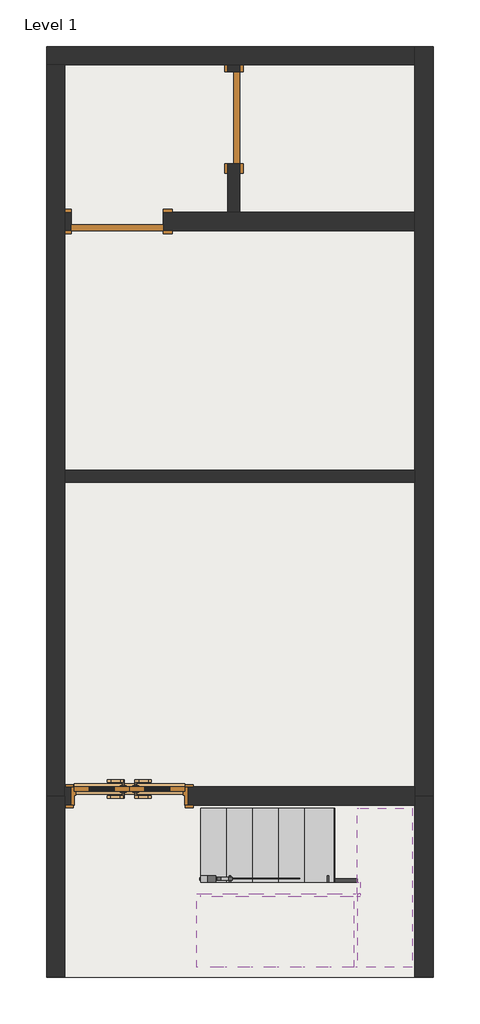
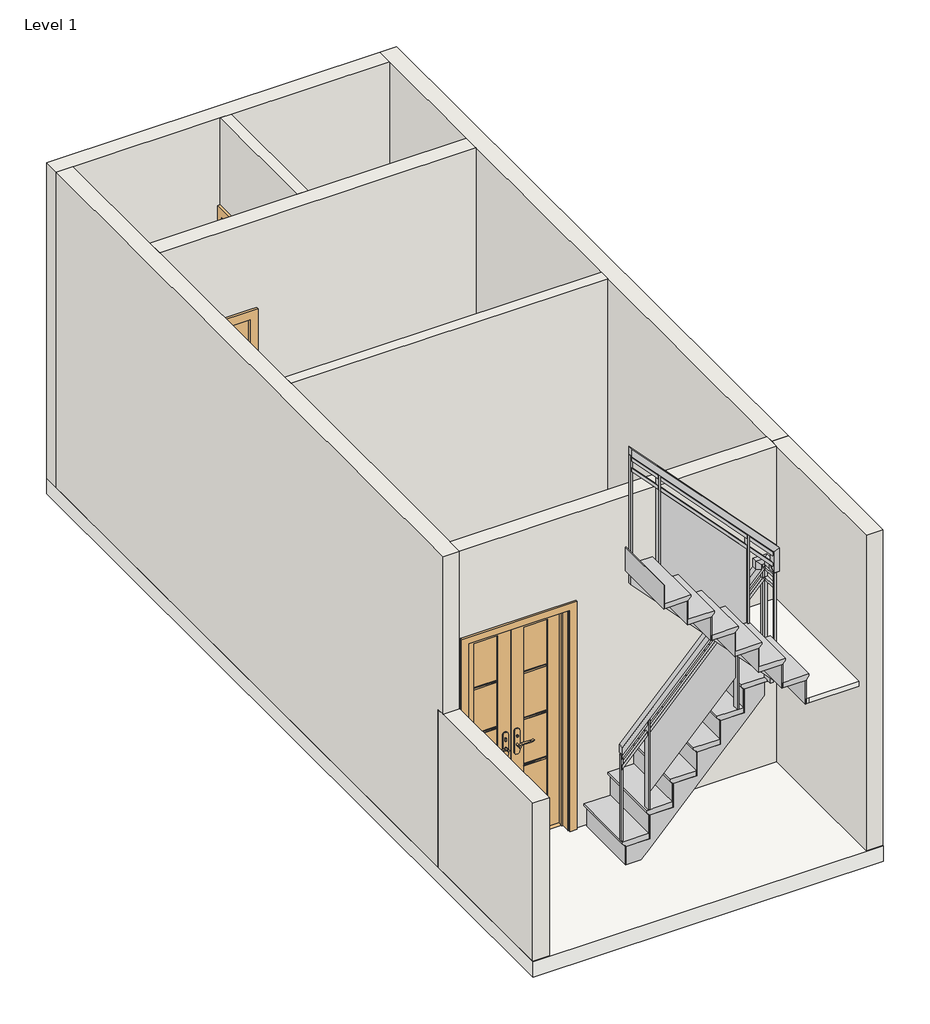
# One storey: 9 walls, 3 doors, 3 members, 2 slabs, 2 stair flights, 1 railing.
"""IFC4 building model written with IfcOpenShell, lengths in millimetres."""

from ifc_helpers import new_model, si_unit, frame, origin, origin_with_axes, place, context, project, spatial, polyline, outline, extrude, faceted_brep, transform, mapped, element, save
from components import door_665efd91, single_flush_2_5_a9addea7, single_flush_2_5_aa9e95e7, non_monolithic_landing_a944a33a, stair_flight_4ab14130, stair_flight_03d0a82c

model = new_model("IFC4")

# Units and contexts
model_context = context("Model", 3, world=origin())
ifc_project = project(units=[si_unit("LENGTHUNIT", "METRE", prefix="MILLI")], contexts=[model_context])

# Site, building, storey
site = spatial("IfcSite", under=ifc_project)
building = spatial("IfcBuilding", under=site)
storey = spatial("IfcBuildingStorey", under=building, Name="Level 1", Elevation=0.0)

# Doors
placement = place(None, origin())
door_shape = door_665efd91(model_context)
element("IfcDoor", 1, ObjectType="Door-Exterior-Double-Full Glass-Wood_Clad : 60\" x 84\"", at=placement, inside=storey, context=model_context, shape_type="MappedRepresentation", body=[
    mapped(door_shape, transform((-5617.280937, -3133.7029636, 0.0), x_axis=(1.0, 0.0, 0.0), y_axis=(0.0, 1.0, 0.0), z_axis=(0.0, 0.0, 1.0))),
])
single_flush_2_5_shape = single_flush_2_5_a9addea7(model_context)
element("IfcDoor", 2, ObjectType="Single-Flush : 2.5'", at=placement, inside=storey, context=model_context, shape_type="MappedRepresentation", body=[
    mapped(single_flush_2_5_shape, transform((-5718.880937, 1617.2335625, 0.0), x_axis=(-1.0, 0.0, 0.0), y_axis=(0.0, -1.0, 0.0), z_axis=(0.0, 0.0, 1.0))),
])
single_flush_2_5_2_shape = single_flush_2_5_aa9e95e7(model_context)
element("IfcDoor", 3, ObjectType="Single-Flush : 2.5'", at=placement, inside=storey, context=model_context, shape_type="MappedRepresentation", body=[
    mapped(single_flush_2_5_2_shape, transform((-4753.680937, 2474.4835625, 0.0), x_axis=(0.0, 1.0, 0.0), y_axis=(-1.0, 0.0, 0.0), z_axis=(0.0, 0.0, 1.0))),
])

# Members
element("IfcMember", 4, ObjectType="Carriage - 2\" Width", at=placement, inside=storey, context=model_context, shape_type="Brep", body=[
    faceted_brep([(-4996.3909298, -3822.6779636, 0.0), (-4861.0694778, -3822.6779636, 0.0), (-4861.0694778, -3848.0779636, 0.0), (-4996.3909298, -3848.0779636, 0.0), (-3732.7409298, -3822.6779636, 1194.7008155), (-3732.7409298, -3848.0779636, 1194.7008155), (-3916.8909298, -3848.0779636, 999.7184625), (-4132.7909298, -3848.0779636, 771.1184625), (-4348.6909298, -3848.0779636, 542.5184625), (-4564.5909298, -3848.0779636, 313.9184625), (-4780.4909298, -3848.0779636, 85.3184625), (-3732.7409298, -3822.6779636, 1320.8), (-4996.3909298, -3822.6779636, 177.8), (-4780.4909298, -3822.6779636, 177.8), (-4780.4909298, -3822.6779636, 406.4), (-4564.5909298, -3822.6779636, 406.4), (-4564.5909298, -3822.6779636, 635.0), (-4348.6909298, -3822.6779636, 635.0), (-4348.6909298, -3822.6779636, 863.6), (-4132.7909298, -3822.6779636, 863.6), (-4132.7909298, -3822.6779636, 1092.2), (-3916.8909298, -3822.6779636, 1092.2), (-3916.8909298, -3822.6779636, 1320.8), (-3916.8909298, -3848.0779636, 1320.8), (-3732.7409298, -3848.0779636, 1320.8), (-3916.8909298, -3848.0779636, 1092.2), (-4132.7909298, -3848.0779636, 1092.2), (-4132.7909298, -3848.0779636, 863.6), (-4348.6909298, -3848.0779636, 863.6), (-4348.6909298, -3848.0779636, 635.0), (-4564.5909298, -3848.0779636, 635.0), (-4564.5909298, -3848.0779636, 406.4), (-4780.4909298, -3848.0779636, 406.4), (-4780.4909298, -3848.0779636, 177.8), (-4996.3909298, -3848.0779636, 177.8)], [[[0, 1, 2, 3]], [[4, 5, 6, 7, 8, 9, 10, 2, 1]], [[11, 4, 1, 0, 12, 13, 14, 15, 16, 17, 18, 19, 20, 21, 22]], [[22, 23, 24, 11]], [[5, 24, 23, 25, 26, 27, 28, 29, 30, 31, 32, 33, 34, 3, 2, 10, 9, 8, 7, 6]], [[34, 12, 0, 3]], [[12, 34, 33, 13]], [[13, 33, 32, 14]], [[14, 32, 31, 15]], [[15, 31, 30, 16]], [[16, 30, 29, 17]], [[17, 29, 28, 18]], [[18, 28, 27, 19]], [[19, 27, 26, 20]], [[20, 26, 25, 21]], [[21, 25, 23, 22]], [[5, 4, 11, 24]]]),
])
element("IfcMember", 5, ObjectType="Carriage - 2\" Width", at=placement, inside=storey, context=model_context, shape_type="Brep", body=[
    faceted_brep([(-5028.1409298, -3945.3664375, 2794.9008155), (-5028.1409298, -3970.7664375, 2794.9008155), (-5028.1409298, -3970.7664375, 2921.0), (-5028.1409298, -3945.3664375, 2921.0), (-3707.3409298, -3970.7664375, 1396.4066978), (-3707.3409298, -3970.7664375, 1549.4), (-3764.4909298, -3970.7664375, 1549.4), (-3764.4909298, -3970.7664375, 1778.0), (-3980.3909298, -3970.7664375, 1778.0), (-3980.3909298, -3970.7664375, 2006.6), (-4196.2909298, -3970.7664375, 2006.6), (-4196.2909298, -3970.7664375, 2235.2), (-4412.1909298, -3970.7664375, 2235.2), (-4412.1909298, -3970.7664375, 2463.8), (-4628.0909298, -3970.7664375, 2463.8), (-4628.0909298, -3970.7664375, 2692.4), (-4843.9909298, -3970.7664375, 2692.4), (-4843.9909298, -3970.7664375, 2921.0), (-4843.9909298, -3945.3664375, 2599.9184625), (-4628.0909298, -3945.3664375, 2371.3184625), (-4412.1909298, -3945.3664375, 2142.7184625), (-4196.2909298, -3945.3664375, 1914.1184625), (-3980.3909298, -3945.3664375, 1685.5184625), (-3764.4909298, -3945.3664375, 1456.9184625), (-3732.7409298, -3945.3664375, 1423.3008155), (-3707.3409298, -3945.3664375, 1396.4066978), (-4843.9909298, -3945.3664375, 2921.0), (-4843.9909298, -3945.3664375, 2692.4), (-4628.0909298, -3945.3664375, 2692.4), (-4628.0909298, -3945.3664375, 2463.8), (-4412.1909298, -3945.3664375, 2463.8), (-4412.1909298, -3945.3664375, 2235.2), (-4196.2909298, -3945.3664375, 2235.2), (-4196.2909298, -3945.3664375, 2006.6), (-3980.3909298, -3945.3664375, 2006.6), (-3980.3909298, -3945.3664375, 1778.0), (-3764.4909298, -3945.3664375, 1778.0), (-3764.4909298, -3945.3664375, 1549.4), (-3732.7409298, -3945.3664375, 1549.4), (-3707.3409298, -3945.3664375, 1549.4)], [[[0, 1, 2, 3]], [[1, 4, 5, 6, 7, 8, 9, 10, 11, 12, 13, 14, 15, 16, 17, 2]], [[1, 0, 18, 19, 20, 21, 22, 23, 24, 25, 4]], [[0, 3, 26, 27, 28, 29, 30, 31, 32, 33, 34, 35, 36, 37, 38, 39, 25, 24, 23, 22, 21, 20, 19, 18]], [[7, 36, 35, 8]], [[36, 7, 6, 37]], [[9, 34, 33, 10]], [[8, 35, 34, 9]], [[11, 32, 31, 12]], [[10, 33, 32, 11]], [[13, 30, 29, 14]], [[12, 31, 30, 13]], [[15, 28, 27, 16]], [[14, 29, 28, 15]], [[17, 26, 3, 2]], [[16, 27, 26, 17]], [[4, 25, 39, 5]], [[37, 6, 5, 39, 38]]]),
])
element("IfcMember", 6, ObjectType="Carriage - 2\" Width", at=placement, inside=storey, context=model_context, shape_type="SweptSolid", body=[
    extrude(outline(polyline([(-3707.3409298, -3945.3664375), (-3732.7409298, -3945.3664375), (-3732.7409298, -3848.0779636), (-3707.3409298, -3848.0779636), (-3707.3409298, -3945.3664375)])), frame((0.0, 0.0, 1371.6), z_axis=(0.0, 0.0, 1.0), x_axis=(1.0, 0.0, 0.0)), (0.0, 0.0, 1.0), 177.8),
])

# Railing
element("IfcRailing", 7, ObjectType="Glass Panel - Bottom Fill", at=placement, inside=storey, context=model_context, shape_type="SolidModel", body=[
    faceted_brep([(-5028.1409298, -3797.2779636, 1143.0), (-5028.1409298, -3797.2779636, 1069.01477), (-5028.1409298, -3848.0779636, 1069.01477), (-5028.1409298, -3848.0779636, 1143.0), (-3808.9409298, -3797.2779636, 2433.9176471), (-3758.1409298, -3797.2779636, 2413.7206524), (-3758.1409298, -3848.0779636, 2413.7206524), (-3808.9409298, -3848.0779636, 2433.9176471), (-3681.9409298, -3945.3664375, 2514.6), (-3732.7409298, -3945.3664375, 2514.6), (-3732.7409298, -3996.1664375, 2463.8), (-3681.9409298, -3996.1664375, 2463.8), (-3681.9409298, -3924.2779636, 2463.8), (-3681.9409298, -3924.2779636, 2514.6), (-3732.7409298, -3924.2779636, 2463.8), (-3732.7409298, -3924.2779636, 2514.6), (-3808.9409298, -3797.2779636, 2514.6), (-3758.1409298, -3797.2779636, 2463.8), (-3758.1409298, -3848.0779636, 2463.8), (-3808.9409298, -3848.0779636, 2514.6), (-3681.9409298, -3797.2779636, 2514.6), (-3681.9409298, -3797.2779636, 2463.8), (-3732.7409298, -3848.0779636, 2463.8), (-3732.7409298, -3848.0779636, 2514.6)], [[[0, 1, 2, 3]], [[1, 0, 4, 5]], [[2, 1, 5, 6]], [[3, 2, 6, 7]], [[0, 3, 7, 4]], [[8, 9, 10, 11]], [[12, 13, 8, 11]], [[14, 12, 11, 10]], [[15, 14, 10, 9]], [[13, 15, 9, 8]], [[5, 4, 16, 17]], [[6, 5, 17, 18]], [[7, 6, 18, 19]], [[4, 7, 19, 16]], [[17, 16, 20, 21]], [[18, 17, 21, 22]], [[19, 18, 22, 23]], [[16, 19, 23, 20]], [[21, 20, 13, 12]], [[22, 21, 12, 14]], [[23, 22, 14, 15]], [[20, 23, 15, 13]]]),
    faceted_brep([(-3681.9409298, -3996.1664375, 2689.4117647), (-3732.7409298, -3996.1664375, 2669.21477), (-3732.7409298, -3945.3664375, 2669.21477), (-3681.9409298, -3945.3664375, 2689.4117647), (-5028.1409298, -3996.1664375, 4114.8), (-5028.1409298, -3945.3664375, 4114.8), (-5028.1409298, -3945.3664375, 4040.81477), (-5028.1409298, -3996.1664375, 4040.81477)], [[[0, 1, 2, 3]], [[4, 5, 6, 7]], [[1, 0, 4, 7]], [[2, 1, 7, 6]], [[3, 2, 6, 5]], [[0, 3, 5, 4]]]),
    faceted_brep([(-3681.9409298, -3945.3664375, 2514.6), (-3681.9409298, -3996.1664375, 2463.8), (-3732.7409298, -3996.1664375, 2463.8), (-3732.7409298, -3945.3664375, 2514.6), (-3681.9409298, -3945.3664375, 2689.4117647), (-3732.7409298, -3945.3664375, 2669.21477), (-3732.7409298, -3996.1664375, 2669.21477), (-3681.9409298, -3996.1664375, 2689.4117647)], [[[0, 1, 2, 3]], [[4, 5, 6, 7]], [[1, 0, 4, 7]], [[2, 1, 7, 6]], [[3, 2, 6, 5]], [[0, 3, 5, 4]]]),
    faceted_brep([(-5028.1409298, -3835.3779636, 1059.8963075), (-5028.1409298, -3809.9779636, 1059.8963075), (-5028.1409298, -3809.9779636, 1022.9036925), (-5028.1409298, -3835.3779636, 1022.9036925), (-3738.2152202, -3835.3779636, 2425.7), (-3738.2152202, -3809.9779636, 2425.7), (-3727.2666394, -3809.9779636, 2400.3), (-3727.2666394, -3835.3779636, 2400.3), (-3720.0409298, -3835.3779636, 2425.7), (-3694.6409298, -3809.9779636, 2425.7), (-3694.6409298, -3809.9779636, 2400.3), (-3720.0409298, -3835.3779636, 2400.3), (-3720.0409298, -3958.0664375, 2425.7), (-3720.0409298, -3958.0664375, 2400.3), (-3694.6409298, -3958.0664375, 2400.3), (-3694.6409298, -3958.0664375, 2425.7)], [[[0, 1, 2, 3]], [[1, 0, 4, 5]], [[2, 1, 5, 6]], [[3, 2, 6, 7]], [[0, 3, 7, 4]], [[5, 4, 8, 9]], [[6, 5, 9, 10]], [[7, 6, 10, 11]], [[4, 7, 11, 8]], [[12, 13, 14, 15]], [[9, 8, 12, 15]], [[10, 9, 15, 14]], [[11, 10, 14, 13]], [[8, 11, 13, 12]]]),
    faceted_brep([(-3694.6409298, -3958.0664375, 2619.755131), (-3694.6409298, -3983.4664375, 2619.755131), (-3694.6409298, -3983.4664375, 2582.762516), (-3694.6409298, -3958.0664375, 2582.762516), (-5028.1409298, -3958.0664375, 4031.6963075), (-5028.1409298, -3958.0664375, 3994.7036925), (-5028.1409298, -3983.4664375, 3994.7036925), (-5028.1409298, -3983.4664375, 4031.6963075)], [[[0, 1, 2, 3]], [[4, 5, 6, 7]], [[1, 0, 4, 7]], [[2, 1, 7, 6]], [[3, 2, 6, 5]], [[0, 3, 5, 4]]]),
    faceted_brep([(-5028.1409298, -3835.3779636, 958.2963075), (-5028.1409298, -3809.9779636, 958.2963075), (-5028.1409298, -3809.9779636, 921.3036925), (-5028.1409298, -3835.3779636, 921.3036925), (-3738.2152202, -3835.3779636, 2324.1), (-3738.2152202, -3809.9779636, 2324.1), (-3727.2666394, -3809.9779636, 2298.7), (-3727.2666394, -3835.3779636, 2298.7), (-3720.0409298, -3835.3779636, 2324.1), (-3694.6409298, -3809.9779636, 2324.1), (-3694.6409298, -3809.9779636, 2298.7), (-3720.0409298, -3835.3779636, 2298.7), (-3720.0409298, -3958.0664375, 2324.1), (-3720.0409298, -3958.0664375, 2298.7), (-3694.6409298, -3958.0664375, 2298.7), (-3694.6409298, -3958.0664375, 2324.1)], [[[0, 1, 2, 3]], [[1, 0, 4, 5]], [[2, 1, 5, 6]], [[3, 2, 6, 7]], [[0, 3, 7, 4]], [[5, 4, 8, 9]], [[6, 5, 9, 10]], [[7, 6, 10, 11]], [[4, 7, 11, 8]], [[12, 13, 14, 15]], [[9, 8, 12, 15]], [[10, 9, 15, 14]], [[11, 10, 14, 13]], [[8, 11, 13, 12]]]),
    faceted_brep([(-3694.6409298, -3958.0664375, 2518.155131), (-3694.6409298, -3983.4664375, 2518.155131), (-3694.6409298, -3983.4664375, 2481.162516), (-3694.6409298, -3958.0664375, 2481.162516), (-5028.1409298, -3958.0664375, 3930.0963075), (-5028.1409298, -3958.0664375, 3893.1036925), (-5028.1409298, -3983.4664375, 3893.1036925), (-5028.1409298, -3983.4664375, 3930.0963075)], [[[0, 1, 2, 3]], [[4, 5, 6, 7]], [[1, 0, 4, 7]], [[2, 1, 7, 6]], [[3, 2, 6, 5]], [[0, 3, 5, 4]]]),
    extrude(outline(polyline([(3765.1500641, -4767.7909298), (3778.597123, -4780.4909298), (2743.2, -4780.4909298), (2743.2, -4767.7909298), (3765.1500641, -4767.7909298)])), frame((0.0, -3996.1664375, 0.0), z_axis=(0.0, 1.0, 0.0), x_axis=(0.0, 0.0, 1.0)), (0.0, 0.0, 1.0), 50.8),
    extrude(outline(polyline([(1957.2941176, -3961.3409298), (2763.5507513, -3961.3409298), (3624.162516, -4774.1409298), (2817.9058824, -4774.1409298), (1957.2941176, -3961.3409298)])), frame((0.0, -3977.3015945, 0.0), z_axis=(0.0, 1.0, 0.0), x_axis=(0.0, 0.0, 1.0)), (0.0, 0.0, 1.0), 6.35),
    extrude(outline(polyline([(2904.5382994, -3954.9909298), (2917.9853582, -3967.6909298), (2057.4, -3967.6909298), (2057.4, -3954.9909298), (2904.5382994, -3954.9909298)])), frame((0.0, -3996.1664375, 0.0), z_axis=(0.0, 1.0, 0.0), x_axis=(0.0, 0.0, 1.0)), (0.0, 0.0, 1.0), 50.8),
    extrude(outline(polyline([(2191.8441818, -3967.6909298), (2178.397123, -3980.3909298), (1143.0, -3980.3909298), (1143.0, -3967.6909298), (2191.8441818, -3967.6909298)])), frame((0.0, -3848.0779636, 0.0), z_axis=(0.0, 1.0, 0.0), x_axis=(0.0, 0.0, 1.0)), (0.0, 0.0, 1.0), 50.8),
    extrude(outline(polyline([(585.6941176, -4786.8409298), (1446.3058824, -3974.0409298), (2037.4095749, -3974.0409298), (1176.7978102, -4786.8409298), (585.6941176, -4786.8409298)])), frame((0.0, -3822.4928066, 0.0), z_axis=(0.0, 1.0, 0.0), x_axis=(0.0, 0.0, 1.0)), (0.0, 0.0, 1.0), 6.35),
    extrude(outline(polyline([(1331.2324171, -4780.4909298), (1317.7853582, -4793.1909298), (457.2, -4793.1909298), (457.2, -4780.4909298), (1331.2324171, -4780.4909298)])), frame((0.0, -3848.0779636, 0.0), z_axis=(0.0, 1.0, 0.0), x_axis=(0.0, 0.0, 1.0)), (0.0, 0.0, 1.0), 50.8),
    extrude(outline(polyline([(-3697.8159298, -3961.2414375), (-3697.8159298, -3980.2914375), (-3716.8659298, -3980.2914375), (-3716.8659298, -3961.2414375), (-3697.8159298, -3961.2414375)])), frame((0.0, 0.0, 1600.2), z_axis=(0.0, 0.0, 1.0), x_axis=(1.0, 0.0, 0.0)), (0.0, 0.0, 1.0), 863.6),
    extrude(outline(polyline([(-3716.8659298, -3832.2029636), (-3716.8659298, -3813.1529636), (-3697.8159298, -3813.1529636), (-3697.8159298, -3832.2029636), (-3716.8659298, -3832.2029636)])), frame((0.0, 0.0, 1600.2), z_axis=(0.0, 0.0, 1.0), x_axis=(1.0, 0.0, 0.0)), (0.0, 0.0, 1.0), 863.6),
    extrude(outline(polyline([(-3742.2659298, -3832.2029636), (-3742.2659298, -3813.1529636), (-3723.2159298, -3813.1529636), (-3723.2159298, -3832.2029636), (-3742.2659298, -3832.2029636)])), frame((0.0, 0.0, 1600.2), z_axis=(0.0, 0.0, 1.0), x_axis=(1.0, 0.0, 0.0)), (0.0, 0.0, 1.0), 863.6),
    extrude(outline(polyline([(4027.3677112, -5015.4409298), (4047.5382994, -5034.4909298), (2971.8, -5034.4909298), (2971.8, -5015.4409298), (4027.3677112, -5015.4409298)])), frame((0.0, -3980.2914375, 0.0), z_axis=(0.0, 1.0, 0.0), x_axis=(0.0, 0.0, 1.0)), (0.0, 0.0, 1.0), 19.05),
    extrude(outline(polyline([(1082.4618288, -5015.4409298), (1062.2912406, -5034.4909298), (228.6, -5034.4909298), (228.6, -5015.4409298), (1082.4618288, -5015.4409298)])), frame((0.0, -3832.2029636, 0.0), z_axis=(0.0, 1.0, 0.0), x_axis=(0.0, 0.0, 1.0)), (0.0, 0.0, 1.0), 19.05),
])

# Slabs
element("IfcSlab", 8, ObjectType="6\"", at=placement, inside=storey, context=model_context, shape_type="SweptSolid", body=[
    extrude(outline(polyline([(-3102.680937, 3065.0335625), (-3102.680937, -4637.5164375), (-6303.080937, -4637.5164375), (-6303.080937, 3065.0335625), (-3102.680937, 3065.0335625)])), frame((0.0, 0.0, -152.4), z_axis=(0.0, 0.0, 1.0), x_axis=(1.0, 0.0, 0.0)), (0.0, 0.0, 1.0), 152.4),
])
non_monolithic_landing_shape = non_monolithic_landing_a944a33a(model_context)
element("IfcSlab", 9, ObjectType="Non-Monolithic Landing", at=placement, inside=storey, context=model_context, shape_type="MappedRepresentation", body=[
    mapped(non_monolithic_landing_shape, transform((0.0, 0.0, 0.0), x_axis=(1.0, 0.0, 0.0), y_axis=(0.0, 1.0, 0.0), z_axis=(0.0, 0.0, 1.0))),
])

# Stair flights
stair_flight_shape = stair_flight_4ab14130(model_context)
element("IfcStairFlight", 10, ObjectType="2\" Tread 1\" Nosing 1/4\" Riser", at=placement, inside=storey, context=model_context, shape_type="MappedRepresentation", body=[
    mapped(stair_flight_shape, transform((0.0, 0.0, 0.0), x_axis=(1.0, 0.0, 0.0), y_axis=(0.0, 1.0, 0.0), z_axis=(0.0, 0.0, 1.0))),
])
stair_flight_2_shape = stair_flight_03d0a82c(model_context)
element("IfcStairFlight", 11, ObjectType="2\" Tread 1\" Nosing 1/4\" Riser", at=placement, inside=storey, context=model_context, shape_type="MappedRepresentation", body=[
    mapped(stair_flight_2_shape, transform((0.0, 0.0, 0.0), x_axis=(1.0, 0.0, 0.0), y_axis=(0.0, 1.0, 0.0), z_axis=(0.0, 0.0, 1.0))),
])

# Walls
element("IfcWall", 12, ObjectType="4\"", at=placement, inside=storey, context=model_context, shape_type="SweptSolid", body=[
    extrude(outline(polyline([(-6150.680937, -440.1664375), (-3255.080937, -440.1664375), (-3255.080937, -541.7664375), (-6150.680937, -541.7664375), (-6150.680937, -440.1664375)])), origin_with_axes(), (0.0, 0.0, 1.0), 3048.0),
])
element("IfcWall", 13, ObjectType="4\"", at=placement, inside=storey, context=model_context, shape_type="SweptSolid", body=[
    extrude(outline(polyline([(2912.6335625, 0.0), (2855.4835625, 0.0), (2855.4835625, 2133.6), (2093.4835625, 2133.6), (2093.4835625, 0.0), (1693.4335625, 0.0), (1693.4335625, 3048.0), (2912.6335625, 3048.0), (2912.6335625, 0.0)])), frame((-4804.480937, 0.0, 0.0), z_axis=(1.0, 0.0, 0.0), x_axis=(0.0, 1.0, 0.0)), (0.0, 0.0, 1.0), 101.6),
])
element("IfcWall", 14, ObjectType="6\"", at=placement, inside=storey, context=model_context, shape_type="Brep", body=[
    faceted_brep([(-6303.080937, 2912.6335625, 0.0), (-6150.680937, 2912.6335625, 0.0), (-4804.480937, 2912.6335625, 0.0), (-4702.880937, 2912.6335625, 0.0), (-3255.080937, 2912.6335625, 0.0), (-3255.080937, 2912.6335625, 3048.0), (-4702.880937, 2912.6335625, 3048.0), (-4804.480937, 2912.6335625, 3048.0), (-6150.680937, 2912.6335625, 3048.0), (-6303.080937, 2912.6335625, 3048.0), (-6303.080937, 3065.0335625, 0.0), (-6303.080937, 3065.0335625, 3048.0), (-3255.080937, 3065.0335625, 3048.0), (-3255.080937, 3065.0335625, 0.0)], [[[0, 1, 2, 3, 4, 5, 6, 7, 8, 9]], [[10, 11, 12, 13]], [[4, 3, 2, 1, 0, 10, 13]], [[9, 8, 7, 6, 5, 12, 11]], [[0, 9, 11, 10]], [[5, 4, 13, 12]]]),
])
element("IfcWall", 15, ObjectType="6\"", at=placement, inside=storey, context=model_context, shape_type="Brep", body=[
    faceted_brep([(-6150.680937, -4631.1664375, 0.0), (-6150.680937, -3213.0779636, 0.0), (-6150.680937, -3136.8779636, 0.0), (-6150.680937, -3136.8779636, 1524.0), (-6150.680937, -3213.0779636, 1524.0), (-6150.680937, -4631.1664375, 1524.0), (-6303.080937, -4631.1664375, 0.0), (-6303.080937, -4631.1664375, 1524.0), (-6303.080937, -3213.0779636, 1524.0), (-6303.080937, -3136.8779636, 1524.0), (-6303.080937, -3136.8779636, 0.0)], [[[0, 1, 2, 3, 4, 5]], [[6, 7, 8, 9, 10]], [[2, 1, 0, 6, 10]], [[3, 2, 10, 9]], [[5, 4, 3, 9, 8, 7]], [[0, 5, 7, 6]]]),
])
element("IfcWall", 16, ObjectType="6\"", at=placement, inside=storey, context=model_context, shape_type="Brep", body=[
    faceted_brep([(-3255.080937, 3065.0335625, 0.0), (-3255.080937, 2912.6335625, 0.0), (-3255.080937, 1693.4335625, 0.0), (-3255.080937, 1541.0335625, 0.0), (-3255.080937, -440.1664375, 0.0), (-3255.080937, -541.7664375, 0.0), (-3255.080937, -3060.6779636, 0.0), (-3255.080937, -3136.8779636, 0.0), (-3255.080937, -3136.8779636, 3048.0), (-3255.080937, -3060.6779636, 3048.0), (-3255.080937, -541.7664375, 3048.0), (-3255.080937, -440.1664375, 3048.0), (-3255.080937, 1541.0335625, 3048.0), (-3255.080937, 1693.4335625, 3048.0), (-3255.080937, 2912.6335625, 3048.0), (-3255.080937, 3065.0335625, 3048.0), (-3102.680937, 3065.0335625, 0.0), (-3102.680937, 3065.0335625, 3048.0), (-3102.680937, -3136.8779636, 3048.0), (-3102.680937, -3136.8779636, 0.0)], [[[0, 1, 2, 3, 4, 5, 6, 7, 8, 9, 10, 11, 12, 13, 14, 15]], [[16, 17, 18, 19]], [[7, 6, 5, 4, 3, 2, 1, 0, 16, 19]], [[8, 7, 19, 18]], [[15, 14, 13, 12, 11, 10, 9, 8, 18, 17]], [[0, 15, 17, 16]]]),
])
element("IfcWall", 17, ObjectType="6\"", at=placement, inside=storey, context=model_context, shape_type="Brep", body=[
    faceted_brep([(-6150.680937, -3060.6779636, 3048.0), (-3255.080937, -3060.6779636, 3048.0), (-3255.080937, -3060.6779636, 0.0), (-5134.680937, -3060.6779636, 0.0), (-5134.680937, -3060.6779636, 2159.0), (-6099.880937, -3060.6779636, 2159.0), (-6099.880937, -3060.6779636, 0.0), (-6150.680937, -3060.6779636, 0.0), (-3255.080937, -3213.0779636, 3048.0), (-6150.680937, -3213.0779636, 3048.0), (-6150.680937, -3213.0779636, 1524.0), (-6150.680937, -3213.0779636, 0.0), (-6099.880937, -3213.0779636, 0.0), (-6099.880937, -3213.0779636, 2159.0), (-5134.680937, -3213.0779636, 2159.0), (-5134.680937, -3213.0779636, 0.0), (-3255.080937, -3213.0779636, 0.0), (-3255.080937, -3136.8779636, 0.0), (-6150.680937, -3136.8779636, 0.0), (-3255.080937, -3136.8779636, 3048.0)], [[[0, 1, 2, 3, 4, 5, 6, 7]], [[8, 9, 10, 11, 12, 13, 14, 15, 16]], [[2, 17, 16, 15, 3]], [[11, 18, 7, 6, 12]], [[1, 0, 9, 8, 19]], [[14, 4, 3, 15]], [[4, 14, 13, 5]], [[5, 13, 12, 6]], [[2, 1, 19, 8, 16, 17]], [[7, 18, 11, 10, 9, 0]]]),
])
element("IfcWall", 18, ObjectType="6\"", at=placement, inside=storey, context=model_context, shape_type="Brep", body=[
    faceted_brep([(-6099.880937, 1693.4335625, 2133.6), (-6099.880937, 1693.4335625, 0.0), (-6150.680937, 1693.4335625, 0.0), (-6150.680937, 1693.4335625, 3048.0), (-4804.480937, 1693.4335625, 3048.0), (-4702.880937, 1693.4335625, 3048.0), (-3255.080937, 1693.4335625, 3048.0), (-3255.080937, 1693.4335625, 0.0), (-4702.880937, 1693.4335625, 0.0), (-4804.480937, 1693.4335625, 0.0), (-5337.880937, 1693.4335625, 0.0), (-5337.880937, 1693.4335625, 2133.6), (-6150.680937, 1541.0335625, 0.0), (-6099.880937, 1541.0335625, 0.0), (-6099.880937, 1541.0335625, 2133.6), (-5337.880937, 1541.0335625, 2133.6), (-5337.880937, 1541.0335625, 0.0), (-3255.080937, 1541.0335625, 0.0), (-3255.080937, 1541.0335625, 3048.0), (-6150.680937, 1541.0335625, 3048.0)], [[[0, 1, 2, 3, 4, 5, 6, 7, 8, 9, 10, 11]], [[12, 13, 14, 15, 16, 17, 18, 19]], [[2, 1, 13, 12]], [[10, 9, 8, 7, 17, 16]], [[6, 5, 4, 3, 19, 18]], [[3, 2, 12, 19]], [[7, 6, 18, 17]], [[14, 13, 1, 0]], [[15, 14, 0, 11]], [[16, 15, 11, 10]]]),
])
element("IfcWall", 19, ObjectType="6\"", at=placement, inside=storey, context=model_context, shape_type="Brep", body=[
    faceted_brep([(-6150.680937, -3136.8779636, 0.0), (-6150.680937, -3060.6779636, 0.0), (-6150.680937, -541.7664375, 0.0), (-6150.680937, -440.1664375, 0.0), (-6150.680937, 1541.0335625, 0.0), (-6150.680937, 1693.4335625, 0.0), (-6150.680937, 2912.6335625, 0.0), (-6150.680937, 2912.6335625, 3048.0), (-6150.680937, 1693.4335625, 3048.0), (-6150.680937, 1541.0335625, 3048.0), (-6150.680937, -440.1664375, 3048.0), (-6150.680937, -541.7664375, 3048.0), (-6150.680937, -3060.6779636, 3048.0), (-6150.680937, -3213.0779636, 3048.0), (-6150.680937, -3213.0779636, 1524.0), (-6150.680937, -3136.8779636, 1524.0), (-6303.080937, -3136.8779636, 0.0), (-6303.080937, -3136.8779636, 1524.0), (-6303.080937, -3213.0779636, 1524.0), (-6303.080937, -3213.0779636, 3048.0), (-6303.080937, 2912.6335625, 3048.0), (-6303.080937, 2912.6335625, 0.0)], [[[0, 1, 2, 3, 4, 5, 6, 7, 8, 9, 10, 11, 12, 13, 14, 15]], [[16, 17, 18, 19, 20, 21]], [[6, 5, 4, 3, 2, 1, 0, 16, 21]], [[13, 12, 11, 10, 9, 8, 7, 20, 19]], [[7, 6, 21, 20]], [[0, 15, 17, 16]], [[14, 18, 17, 15]], [[14, 13, 19, 18]]]),
])
element("IfcWall", 20, ObjectType="6\"", at=placement, inside=storey, context=model_context, shape_type="Brep", body=[
    faceted_brep([(-3255.080937, -3136.8779636, 0.0), (-3255.080937, -3213.0779636, 0.0), (-3255.080937, -4631.1664375, 0.0), (-3255.080937, -4631.1664375, 3048.0), (-3255.080937, -3213.0779636, 3048.0), (-3255.080937, -3136.8779636, 3048.0), (-3102.680937, -3136.8779636, 0.0), (-3102.680937, -3136.8779636, 3048.0), (-3102.680937, -4631.1664375, 3048.0), (-3102.680937, -4631.1664375, 0.0)], [[[0, 1, 2, 3, 4, 5]], [[6, 7, 8, 9]], [[2, 1, 0, 6, 9]], [[3, 2, 9, 8]], [[5, 4, 3, 8, 7]], [[0, 5, 7, 6]]]),
])

save(model, "model.ifc")

# Revit data of these elements
# Type "Door-Exterior-Double-Full Glass-Wood_Clad : 60\" x 84\""
#   Type Mark = "8"
#   Assembly Code = "B2030100"
#   Analytic Construction = "French door, wood frame with double glass"
#   Top Rail = 0' - 4 11/16"
#   Threshold Offset [instance default] = 0' - 0 1/2"
#   Thickness = 0' - 1 3/8"
#   Thermal Resistance (R) = 1.9158 (h·ft²·°F)/BTU
#   Swing Angle [instance default] = 90.00°
#   Stiles = 0' - 4 3/4"
#   Rough Width = 3' - 2"
#   Rough Height = 7' - 1"
#   Panel Width = 1' - 6"
#   Door Offset [instance default] = 0' - 0"
#   Height = 7' - 0"
#   Width = 3' - 0"
#   Heat Transfer Coefficient (U) = 0.5220 BTU/(h·ft²·°F)
#   Bottom Rail = 0' - 9 1/8"
#   Exterior Trim [instance default] = yes
#   Threshold [instance default] = yes
#   Show Grill [instance default] = yes
#   Function = 1
#   Trim Material = Cherry
#   Threshold Material = Cherry
#   Panel Material = Cherry
#   Glazing = Glass
#   Frame Material = Cherry
#   Door Handle Material = Aluminum
#   Visual Light Transmittance = 0
#   Solar Heat Gain Coefficient = 0
#   Wall Closure = (empty or 0)
#   Construction Type = (empty or 0)
# Type "Single-Flush : 2.5'"
#   Type Mark = "9"
#   Construction Type Id = "MDOOR"
#   Assembly Code = "C1020"
#   Analytic Construction = "Metal"
#   Thickness = 0' - 2"
#   Heat Transfer Coefficient (U) = 0.651978 BTU/(h·ft²·°F)
#   Height = 7' - 0"
#   Trim Projection Ext = 0' - 1"
#   Trim Projection Int = 0' - 1"
#   Trim Width = 0' - 3"
#   Width = 2' - 6"
#   Define Thermal Properties by = 1
#   Door Material = Door - Panel
#   Frame Material = Door - Frame
#   Visual Light Transmittance = 0
#   Solar Heat Gain Coefficient = 0
#   Function = (empty or 0)
#   Wall Closure = (empty or 0)
# Type "Glass Panel - Bottom Fill"
#   Assembly Code = "C2010400"
#   built-in parameter 1008612 = 0.0416667 (stored number, unit not read)
#   built-in parameter 1008611 = 0.0416667 (stored number, unit not read)
#   built-in parameter 1008609 = 0.333333 (stored number, unit not read)
#   built-in parameter 1008604 = 0.166667 (stored number, unit not read)
#   built-in parameter 1008603 = 0.166667 (stored number, unit not read)
#   Railing Height = 3' - 0"
#   built-in parameter 1008630 = 2
#   built-in parameter 1008610 = 2
#   built-in parameter 1008618 = Baluster - Square : 3/4"
# Type "6\""
#   Assembly Code = "B1010"
#   Function = 0
#   Layers, outside or top first: 0' - 6" no material (function 1)
# Type "4\""
#   Assembly Code = "B2010"
#   Layers, outside or top first: 0' - 4" no material (function 1)
# Type "6\""
#   Assembly Code = "B2010"
#   Layers, outside or top first: 0' - 6" no material (function 1)
# Element 1 (IfcDoor, "Door-Exterior-Double-Full Glass-Wood_Clad : 60\" x 84\"")
#   Threshold Offset = 0' - 0 1/2"
#   Swing Angle = 90.00°
#   Door Offset = 0' - 0"
#   Threshold = yes
#   Show Grill = yes
#   Exterior Trim = yes
#   Phase Created = New Construction
#   Materials on its faces: "Cherry", "Aluminum", "Glass"
# Elements 2, 3 (IfcDoor, "Single-Flush : 2.5'")
#   Phase Created = New Construction
#   Materials on its faces: "Door - Frame", "Door - Panel"
# Elements 4, 5, 6 (IfcMember, "Carriage - 2\" Width")
#   Phase Created = New Construction
# Element 7 (IfcRailing, "Glass Panel - Bottom Fill")
#   Phase Created = New Construction
#   Materials on its faces: "Glass"
# Element 8 (IfcSlab, "6\"")
#   Height Offset From Level = 0' - 0"
#   Phase Created = New Construction
#   Materials on its faces: "Default Floor"
# Element 9 (IfcSlab, "Non-Monolithic Landing")
#   Phase Created = New Construction
# Elements 10, 11 (IfcStairFlight, "2\" Tread 1\" Nosing 1/4\" Riser")
#   Phase Created = New Construction
# Elements 12, 13 (IfcWall, "4\"")
#   Top Offset = 0' - 0"
#   Base Offset = 0' - 0"
#   Unconnected Height = 10' - 0"
#   wall height = 10' - 0"
#   Phase Created = New Construction
#   Base Constraint = Level 1
#   Materials on its faces: "Default Wall"
# Elements 14, 16, 17, 18, 19, 20 (IfcWall, "6\"")
#   Top Offset = 0' - 0"
#   Base Offset = 0' - 0"
#   Unconnected Height = 10' - 0"
#   wall height = 10' - 0"
#   Phase Created = New Construction
#   Base Constraint = Level 1
#   Materials on its faces: "Default Wall"
# Element 15 (IfcWall, "6\"")
#   Top Offset = 0' - 0"
#   Base Offset = 0' - 0"
#   Unconnected Height = 5' - 0"
#   wall height = 5' - 0"
#   Phase Created = New Construction
#   Base Constraint = Level 1
#   Materials on its faces: "Default Wall"
# Materials
#   "Cherry": class "Wood", colour RGB 226 177 128, transparency 0, Description = "Prunus Serotina", Cost = 0
#   "Glass": class "Glass", colour RGB 0 128 192, transparency 0.75, Description = "Soda Lime Glass", Cost = 0
#   "Aluminum": class "Metal", colour RGB 247 247 247, transparency 0, Description = "Aluminum 6061", Cost = 0
#   "Door - Panel": class "Wood", colour RGB 210 159 95, transparency 0
#   "Door - Frame": colour RGB 118 70 51, transparency 0
#   "Default Floor": colour RGB 128 128 128, transparency 0
#   "Default Wall": colour RGB 128 128 128, transparency 0
